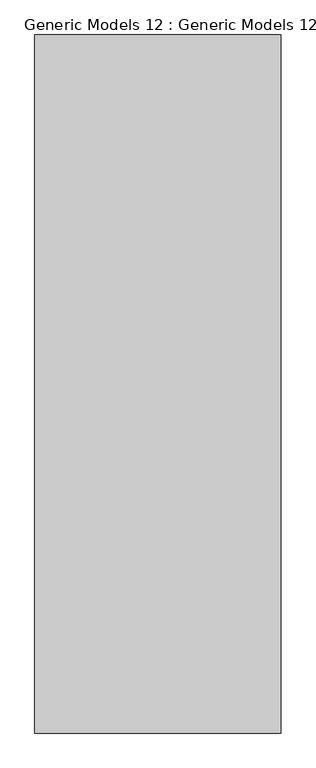
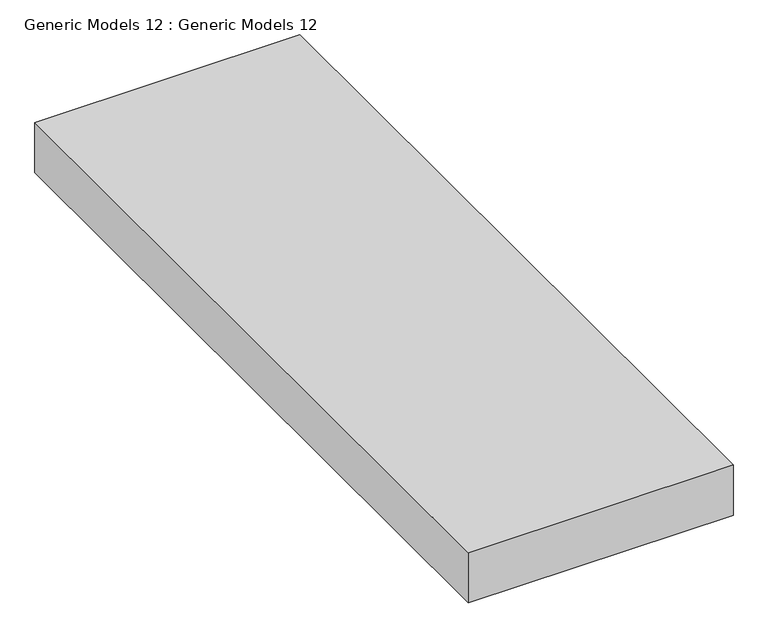
"""IFC4 building model written with IfcOpenShell, lengths in millimetres: proxy geometry, Generic Models 12 : Generic Models 12."""

from ifc_helpers import new_model, si_unit, frame, origin, place, context, project, spatial, polyline, outline, extrude, source, transform, mapped, element, save


def generic_models_12_generic_models_12_5e433632(model_context):
    return source(origin(), model_context, "Body", "SweptSolid", [
        extrude(outline(polyline([(-16985.0859258, 353.6460165), (-16223.0859258, 353.6460165), (-16223.0859258, -1806.1165273), (-16985.0859258, -1806.1165273), (-16985.0859258, 353.6460165)])), frame((0.0, 0.0, 2325.7757409), z_axis=(0.0, 0.0, 1.0), x_axis=(1.0, 0.0, 0.0)), (0.0, 0.0, 1.0), 152.4),
    ])


if __name__ == "__main__":
    model = new_model("IFC4")
    model_context = context("Model", 3, world=origin())
    ifc_project = project(units=[si_unit("LENGTHUNIT", "METRE", prefix="MILLI")], contexts=[model_context])
    site = spatial("IfcSite", under=ifc_project)
    building = spatial("IfcBuilding", under=site)
    placement = place(None, origin())
    generic_models_12_generic_models_12_shape = generic_models_12_generic_models_12_5e433632(model_context)
    element("IfcBuildingElementProxy", 1, Name="Generic Models 12 : Generic Models 12", ObjectType="Generic Models 12 : Generic Models 12", at=placement, inside=building, context=model_context, shape_type="MappedRepresentation", body=[
        mapped(generic_models_12_generic_models_12_shape, transform((0.0, 0.0, 0.0), x_axis=(1.0, 0.0, 0.0), y_axis=(0.0, 1.0, 0.0), z_axis=(0.0, 0.0, 1.0))),
    ])
    save(model, "model.ifc")
